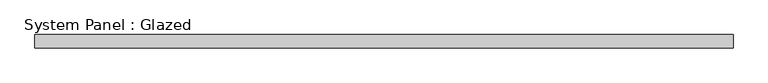
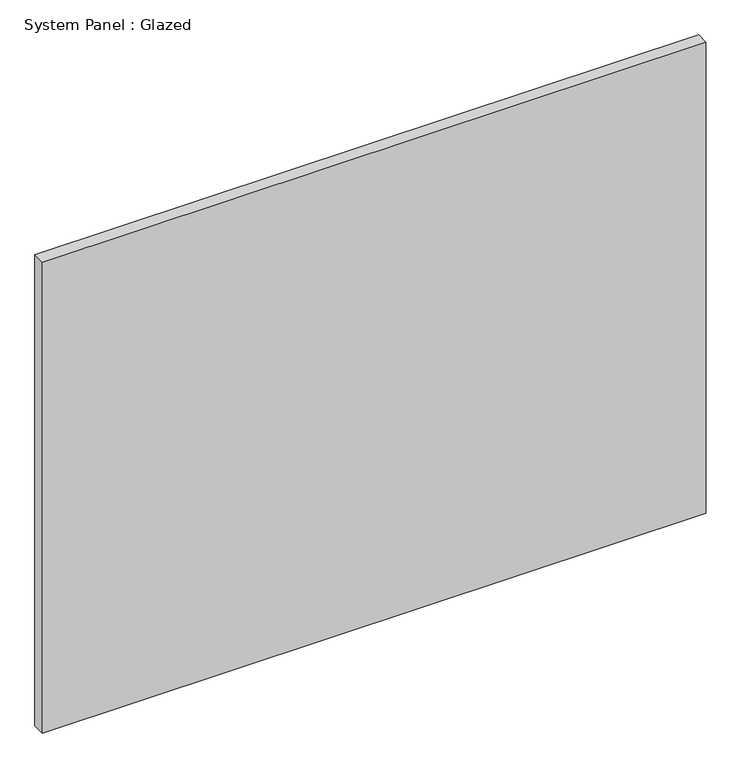
"""IFC4 building model written with IfcOpenShell, lengths in millimetres: plate geometry, System Panel : Glazed."""

from ifc_helpers import new_model, si_unit, origin, origin_with_axes, place, context, project, spatial, polyline, outline, extrude, source, transform, mapped, element, save


def system_panel_glazed_c3157265(model_context):
    return source(origin(), model_context, "Body", "SweptSolid", [
        extrude(outline(polyline([(661.32075, 19.05), (-661.32075, 19.05), (-661.32075, 44.45), (661.32075, 44.45), (661.32075, 19.05)])), origin_with_axes(), (0.0, 0.0, 1.0), 992.4415),
    ])


if __name__ == "__main__":
    model = new_model("IFC4")
    model_context = context("Model", 3, world=origin())
    ifc_project = project(units=[si_unit("LENGTHUNIT", "METRE", prefix="MILLI")], contexts=[model_context])
    site = spatial("IfcSite", under=ifc_project)
    building = spatial("IfcBuilding", under=site)
    placement = place(None, origin())
    system_panel_glazed_shape = system_panel_glazed_c3157265(model_context)
    element("IfcPlate", 1, ObjectType="System Panel : Glazed", at=placement, inside=building, context=model_context, shape_type="MappedRepresentation", body=[
        mapped(system_panel_glazed_shape, transform((0.0, 0.0, 0.0), x_axis=(1.0, 0.0, 0.0), y_axis=(0.0, 1.0, 0.0), z_axis=(0.0, 0.0, 1.0))),
    ])
    save(model, "model.ifc")

# Revit data of these elements
# Type "System Panel : Glazed"
#   Construction Type Id = "GSP4R"
#   Analytic Construction = "1/8 in Pilkington single glazing"
#   Visual Light Transmittance = 0.9
#   Solar Heat Gain Coefficient = 0.86
#   Heat Transfer Coefficient (U) = 1.18115 BTU/(h·ft²·°F)
#   Define Thermal Properties by = 1
# Element 1 (IfcPlate, "System Panel : Glazed")
#   Materials on its faces: "Glass"
# Materials
#   "Glass": class "Glass", colour RGB 0 128 192, transparency 0.75, Description = "Soda Lime Glass", Cost = 0
